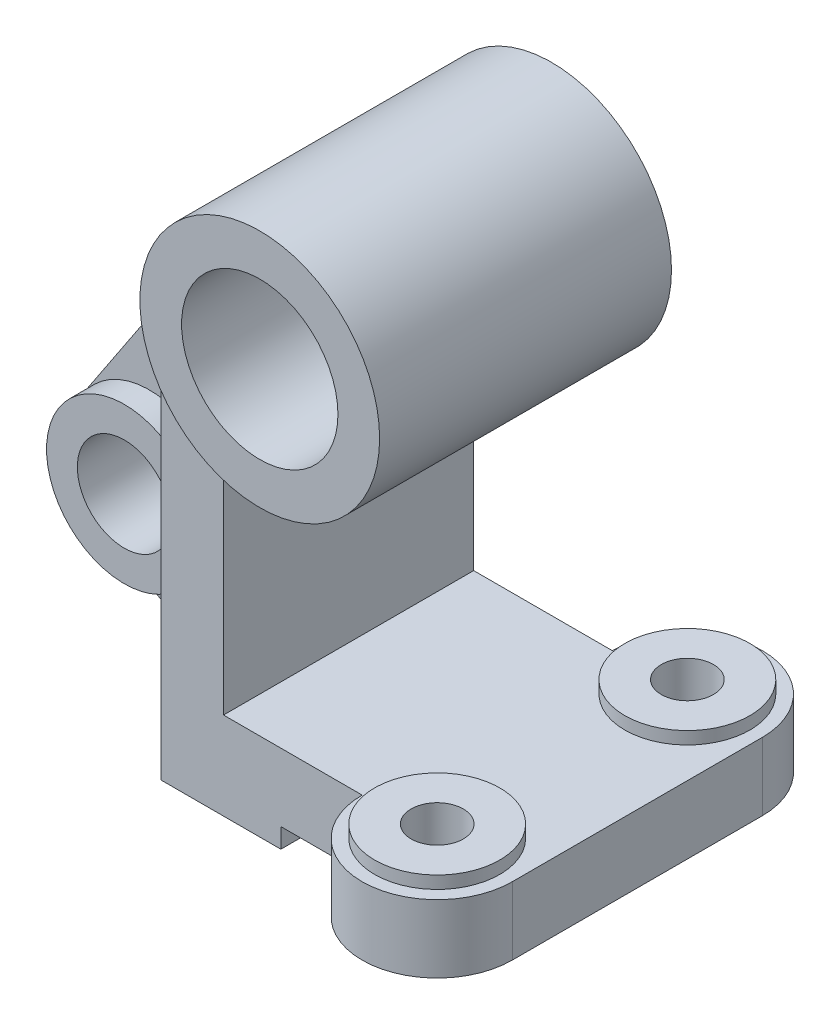
ISO-10303-21;
HEADER;
FILE_DESCRIPTION(('STEP AP214'),'2;1');
FILE_NAME('part.step','',(''),(''),'','','');
FILE_SCHEMA(('AUTOMOTIVE_DESIGN { 1 0 10303 214 1 1 1 1 }'));
ENDSEC;
DATA;
#1=APPLICATION_CONTEXT('core data for automotive mechanical design processes');
#2=APPLICATION_PROTOCOL_DEFINITION('international standard','automotive_design',2000,#1);
#3=PRODUCT_CONTEXT('',#1,'mechanical');
#4=PRODUCT('Part','Part','',(#3));
#5=PRODUCT_RELATED_PRODUCT_CATEGORY('part','',(#4));
#6=PRODUCT_DEFINITION_FORMATION('','',#4);
#7=PRODUCT_DEFINITION_CONTEXT('part definition',#1,'design');
#8=PRODUCT_DEFINITION('design','',#6,#7);
#9=PRODUCT_DEFINITION_SHAPE('','',#8);
#10=(LENGTH_UNIT() NAMED_UNIT(*) SI_UNIT(.MILLI.,.METRE.));
#11=(NAMED_UNIT(*) PLANE_ANGLE_UNIT() SI_UNIT($,.RADIAN.));
#12=(NAMED_UNIT(*) SI_UNIT($,.STERADIAN.) SOLID_ANGLE_UNIT());
#13=UNCERTAINTY_MEASURE_WITH_UNIT(LENGTH_MEASURE(1.E-05),#10,'distance_accuracy_value','');
#14=(GEOMETRIC_REPRESENTATION_CONTEXT(3) GLOBAL_UNCERTAINTY_ASSIGNED_CONTEXT((#13)) GLOBAL_UNIT_ASSIGNED_CONTEXT((#10,
#11,#12)) REPRESENTATION_CONTEXT('',''));
#15=CARTESIAN_POINT('',(0.,0.,0.));
#16=DIRECTION('',(0.,0.,1.));
#17=DIRECTION('',(1.,0.,0.));
#18=AXIS2_PLACEMENT_3D('',#15,#16,#17);
#19=CARTESIAN_POINT('',(67.1412556053812,0.,60.));
#20=DIRECTION('',(0.,1.,0.));
#21=DIRECTION('',(0.,0.,1.));
#22=AXIS2_PLACEMENT_3D('',#19,#20,#21);
#23=PLANE('',#22);
#24=DIRECTION('',(0.,0.,-1.));
#25=VECTOR('',#24,1.);
#26=CARTESIAN_POINT('',(-7.8587443946188,0.,145.));
#27=LINE('',#26,#25);
#28=CARTESIAN_POINT('',(-7.8587443946188,0.,60.));
#29=VERTEX_POINT('',#28);
#30=CARTESIAN_POINT('',(-7.8587443946188,0.,-60.));
#31=VERTEX_POINT('',#30);
#32=EDGE_CURVE('E160',#29,#31,#27,.T.);
#33=ORIENTED_EDGE('',*,*,#32,.F.);
#34=DIRECTION('',(1.,0.,0.));
#35=VECTOR('',#34,1.);
#36=CARTESIAN_POINT('',(-65.3587443946188,0.,60.));
#37=LINE('',#36,#35);
#38=CARTESIAN_POINT('',(-65.3587443946188,0.,60.));
#39=VERTEX_POINT('',#38);
#40=EDGE_CURVE('E317',#39,#29,#37,.T.);
#41=ORIENTED_EDGE('',*,*,#40,.F.);
#42=DIRECTION('',(0.,0.,1.));
#43=VECTOR('',#42,1.);
#44=CARTESIAN_POINT('',(-65.3587443946188,0.,-60.));
#45=LINE('',#44,#43);
#46=CARTESIAN_POINT('',(-65.3587443946188,0.,13.));
#47=VERTEX_POINT('',#46);
#48=EDGE_CURVE('E297',#47,#39,#45,.T.);
#49=ORIENTED_EDGE('',*,*,#48,.F.);
#50=DIRECTION('',(0.,0.,-1.));
#51=VECTOR('',#50,1.);
#52=CARTESIAN_POINT('',(-65.3587443946188,0.,13.));
#53=LINE('',#52,#51);
#54=CARTESIAN_POINT('',(-65.3587443946188,0.,-13.));
#55=VERTEX_POINT('',#54);
#56=EDGE_CURVE('E250',#47,#55,#53,.T.);
#57=ORIENTED_EDGE('',*,*,#56,.T.);
#58=CARTESIAN_POINT('',(-65.3587443946188,0.,-60.));
#59=VERTEX_POINT('',#58);
#60=EDGE_CURVE('E312',#59,#55,#45,.T.);
#61=ORIENTED_EDGE('',*,*,#60,.F.);
#62=DIRECTION('',(-1.,0.,0.));
#63=VECTOR('',#62,1.);
#64=CARTESIAN_POINT('',(-65.3587443946188,0.,-60.));
#65=LINE('',#64,#63);
#66=EDGE_CURVE('E302',#31,#59,#65,.T.);
#67=ORIENTED_EDGE('',*,*,#66,.F.);
#68=EDGE_LOOP('',(#33,#41,#49,#57,#61,#67));
#69=FACE_BOUND('',#68,.T.);
#70=ADVANCED_FACE('F41',(#69),#23,.F.);
#71=CARTESIAN_POINT('',(-65.3587443946188,42.,60.));
#72=DIRECTION('',(0.,0.,-1.));
#73=DIRECTION('',(-1.,0.,0.));
#74=AXIS2_PLACEMENT_3D('',#71,#72,#73);
#75=PLANE('',#74);
#76=DIRECTION('',(0.,-1.,0.));
#77=VECTOR('',#76,1.);
#78=CARTESIAN_POINT('',(-7.8587443946188,42.,60.));
#79=LINE('',#78,#77);
#80=CARTESIAN_POINT('',(-7.8587443946188,9.41903160837437,60.));
#81=VERTEX_POINT('',#80);
#82=EDGE_CURVE('E201',#81,#29,#79,.T.);
#83=ORIENTED_EDGE('',*,*,#82,.F.);
#84=DIRECTION('',(-1.,0.,0.));
#85=VECTOR('',#84,1.);
#86=CARTESIAN_POINT('',(-65.3587443946188,9.41903160837437,60.));
#87=LINE('',#86,#85);
#88=CARTESIAN_POINT('',(31.1412556053812,9.41903160837437,60.));
#89=VERTEX_POINT('',#88);
#90=EDGE_CURVE('E166',#89,#81,#87,.T.);
#91=ORIENTED_EDGE('',*,*,#90,.F.);
#92=DIRECTION('',(0.,-1.,0.));
#93=VECTOR('',#92,1.);
#94=CARTESIAN_POINT('',(31.1412556053812,42.,60.));
#95=LINE('',#94,#93);
#96=CARTESIAN_POINT('',(31.1412556053812,42.,60.));
#97=VERTEX_POINT('',#96);
#98=EDGE_CURVE('E170',#97,#89,#95,.T.);
#99=ORIENTED_EDGE('',*,*,#98,.F.);
#100=DIRECTION('',(1.,0.,0.));
#101=VECTOR('',#100,1.);
#102=CARTESIAN_POINT('',(-65.3587443946188,42.,60.));
#103=LINE('',#102,#101);
#104=CARTESIAN_POINT('',(-35.3587443946188,42.,60.));
#105=VERTEX_POINT('',#104);
#106=EDGE_CURVE('E301',#105,#97,#103,.T.);
#107=ORIENTED_EDGE('',*,*,#106,.F.);
#108=DIRECTION('',(0.,-1.,0.));
#109=VECTOR('',#108,1.);
#110=CARTESIAN_POINT('',(-35.3587443946188,208.,60.));
#111=LINE('',#110,#109);
#112=CARTESIAN_POINT('',(-35.3587443946188,153.774019557073,60.));
#113=VERTEX_POINT('',#112);
#114=EDGE_CURVE('E296',#113,#105,#111,.T.);
#115=ORIENTED_EDGE('',*,*,#114,.F.);
#116=CARTESIAN_POINT('',(-7.9756626414212,204.335040449631,60.));
#117=DIRECTION('',(0.,0.,-1.));
#118=DIRECTION('',(-1.,0.,0.));
#119=AXIS2_PLACEMENT_3D('',#116,#117,#118);
#120=CIRCLE('',#119,57.5);
#121=CARTESIAN_POINT('',(-65.3587443946188,200.670080899262,60.));
#122=VERTEX_POINT('',#121);
#123=EDGE_CURVE('E290',#122,#113,#120,.F.);
#124=ORIENTED_EDGE('',*,*,#123,.F.);
#125=DIRECTION('',(0.,-1.,0.));
#126=VECTOR('',#125,1.);
#127=CARTESIAN_POINT('',(-65.3587443946188,42.,60.));
#128=LINE('',#127,#126);
#129=EDGE_CURVE('E172',#122,#39,#128,.T.);
#130=ORIENTED_EDGE('',*,*,#129,.T.);
#131=ORIENTED_EDGE('',*,*,#40,.T.);
#132=EDGE_LOOP('',(#83,#91,#99,#107,#115,#124,#130,#131));
#133=FACE_BOUND('',#132,.T.);
#134=ADVANCED_FACE('F336',(#133),#75,.F.);
#135=CARTESIAN_POINT('',(67.1412556053812,42.,60.));
#136=DIRECTION('',(0.,-1.,0.));
#137=DIRECTION('',(0.,0.,-1.));
#138=AXIS2_PLACEMENT_3D('',#135,#136,#137);
#139=CYLINDRICAL_SURFACE('',#138,36.);
#140=CARTESIAN_POINT('',(67.1412556053812,9.41903160837437,60.));
#141=DIRECTION('',(0.,-1.,0.));
#142=DIRECTION('',(0.,0.,-1.));
#143=AXIS2_PLACEMENT_3D('',#140,#141,#142);
#144=CIRCLE('',#143,36.);
#145=CARTESIAN_POINT('',(103.141255605381,9.41903160837437,60.));
#146=VERTEX_POINT('',#145);
#147=EDGE_CURVE('E148',#146,#89,#144,.T.);
#148=ORIENTED_EDGE('',*,*,#147,.F.);
#149=DIRECTION('',(0.,-1.,0.));
#150=VECTOR('',#149,1.);
#151=CARTESIAN_POINT('',(103.141255605381,42.,60.));
#152=LINE('',#151,#150);
#153=CARTESIAN_POINT('',(103.141255605381,42.,60.));
#154=VERTEX_POINT('',#153);
#155=EDGE_CURVE('E165',#154,#146,#152,.T.);
#156=ORIENTED_EDGE('',*,*,#155,.F.);
#157=CARTESIAN_POINT('',(67.1412556053812,42.,60.));
#158=DIRECTION('',(0.,1.,0.));
#159=DIRECTION('',(0.,0.,1.));
#160=AXIS2_PLACEMENT_3D('',#157,#158,#159);
#161=CIRCLE('',#160,36.);
#162=EDGE_CURVE('E303',#97,#154,#161,.T.);
#163=ORIENTED_EDGE('',*,*,#162,.F.);
#164=ORIENTED_EDGE('',*,*,#98,.T.);
#165=EDGE_LOOP('',(#148,#156,#163,#164));
#166=FACE_BOUND('',#165,.T.);
#167=ADVANCED_FACE('F162',(#166),#139,.T.);
#168=CARTESIAN_POINT('',(103.141255605381,42.,-60.));
#169=DIRECTION('',(-1.,0.,0.));
#170=DIRECTION('',(0.,0.,1.));
#171=AXIS2_PLACEMENT_3D('',#168,#169,#170);
#172=PLANE('',#171);
#173=DIRECTION('',(0.,0.,-1.));
#174=VECTOR('',#173,1.);
#175=CARTESIAN_POINT('',(103.141255605381,9.41903160837437,145.));
#176=LINE('',#175,#174);
#177=CARTESIAN_POINT('',(103.141255605381,9.41903160837437,-60.));
#178=VERTEX_POINT('',#177);
#179=EDGE_CURVE('E149',#146,#178,#176,.T.);
#180=ORIENTED_EDGE('',*,*,#179,.T.);
#181=DIRECTION('',(0.,-1.,0.));
#182=VECTOR('',#181,1.);
#183=CARTESIAN_POINT('',(103.141255605381,42.,-60.));
#184=LINE('',#183,#182);
#185=CARTESIAN_POINT('',(103.141255605381,42.,-60.));
#186=VERTEX_POINT('',#185);
#187=EDGE_CURVE('E175',#186,#178,#184,.T.);
#188=ORIENTED_EDGE('',*,*,#187,.F.);
#189=DIRECTION('',(0.,0.,-1.));
#190=VECTOR('',#189,1.);
#191=CARTESIAN_POINT('',(103.141255605381,42.,-60.));
#192=LINE('',#191,#190);
#193=EDGE_CURVE('E171',#154,#186,#192,.T.);
#194=ORIENTED_EDGE('',*,*,#193,.F.);
#195=ORIENTED_EDGE('',*,*,#155,.T.);
#196=EDGE_LOOP('',(#180,#188,#194,#195));
#197=FACE_BOUND('',#196,.T.);
#198=ADVANCED_FACE('F167',(#197),#172,.F.);
#199=CARTESIAN_POINT('',(67.1412556053812,42.,-60.));
#200=DIRECTION('',(0.,-1.,0.));
#201=DIRECTION('',(0.,0.,-1.));
#202=AXIS2_PLACEMENT_3D('',#199,#200,#201);
#203=CYLINDRICAL_SURFACE('',#202,36.);
#204=CARTESIAN_POINT('',(67.1412556053812,9.41903160837437,-60.));
#205=DIRECTION('',(0.,-1.,0.));
#206=DIRECTION('',(0.,0.,-1.));
#207=AXIS2_PLACEMENT_3D('',#204,#205,#206);
#208=CIRCLE('',#207,36.);
#209=CARTESIAN_POINT('',(31.1412556053812,9.41903160837437,-60.));
#210=VERTEX_POINT('',#209);
#211=EDGE_CURVE('E155',#210,#178,#208,.T.);
#212=ORIENTED_EDGE('',*,*,#211,.F.);
#213=DIRECTION('',(0.,-1.,0.));
#214=VECTOR('',#213,1.);
#215=CARTESIAN_POINT('',(31.1412556053812,42.,-60.));
#216=LINE('',#215,#214);
#217=CARTESIAN_POINT('',(31.1412556053812,42.,-60.));
#218=VERTEX_POINT('',#217);
#219=EDGE_CURVE('E176',#218,#210,#216,.T.);
#220=ORIENTED_EDGE('',*,*,#219,.F.);
#221=CARTESIAN_POINT('',(67.1412556053812,42.,-60.));
#222=DIRECTION('',(0.,1.,0.));
#223=DIRECTION('',(0.,0.,-1.));
#224=AXIS2_PLACEMENT_3D('',#221,#222,#223);
#225=CIRCLE('',#224,36.);
#226=EDGE_CURVE('E310',#186,#218,#225,.T.);
#227=ORIENTED_EDGE('',*,*,#226,.F.);
#228=ORIENTED_EDGE('',*,*,#187,.T.);
#229=EDGE_LOOP('',(#212,#220,#227,#228));
#230=FACE_BOUND('',#229,.T.);
#231=ADVANCED_FACE('F327',(#230),#203,.T.);
#232=CARTESIAN_POINT('',(-65.3587443946188,42.,-60.));
#233=DIRECTION('',(0.,0.,1.));
#234=DIRECTION('',(1.,0.,0.));
#235=AXIS2_PLACEMENT_3D('',#232,#233,#234);
#236=PLANE('',#235);
#237=DIRECTION('',(0.,1.,0.));
#238=VECTOR('',#237,1.);
#239=CARTESIAN_POINT('',(-7.8587443946188,42.,-60.));
#240=LINE('',#239,#238);
#241=CARTESIAN_POINT('',(-7.8587443946188,9.41903160837437,-60.));
#242=VERTEX_POINT('',#241);
#243=EDGE_CURVE('E11',#31,#242,#240,.T.);
#244=ORIENTED_EDGE('',*,*,#243,.F.);
#245=ORIENTED_EDGE('',*,*,#66,.T.);
#246=DIRECTION('',(0.,-1.,0.));
#247=VECTOR('',#246,1.);
#248=CARTESIAN_POINT('',(-65.3587443946188,42.,-60.));
#249=LINE('',#248,#247);
#250=CARTESIAN_POINT('',(-65.3587443946188,200.670080899262,-60.));
#251=VERTEX_POINT('',#250);
#252=EDGE_CURVE('E315',#251,#59,#249,.T.);
#253=ORIENTED_EDGE('',*,*,#252,.F.);
#254=CARTESIAN_POINT('',(-7.9756626414212,204.335040449631,-60.));
#255=DIRECTION('',(0.,0.,1.));
#256=DIRECTION('',(1.,0.,0.));
#257=AXIS2_PLACEMENT_3D('',#254,#255,#256);
#258=CIRCLE('',#257,57.5);
#259=CARTESIAN_POINT('',(-35.3587443946188,153.774019557073,-60.));
#260=VERTEX_POINT('',#259);
#261=EDGE_CURVE('E282',#260,#251,#258,.F.);
#262=ORIENTED_EDGE('',*,*,#261,.F.);
#263=DIRECTION('',(0.,-1.,0.));
#264=VECTOR('',#263,1.);
#265=CARTESIAN_POINT('',(-35.3587443946188,208.,-60.));
#266=LINE('',#265,#264);
#267=CARTESIAN_POINT('',(-35.3587443946188,42.,-60.));
#268=VERTEX_POINT('',#267);
#269=EDGE_CURVE('E298',#260,#268,#266,.T.);
#270=ORIENTED_EDGE('',*,*,#269,.T.);
#271=DIRECTION('',(-1.,0.,0.));
#272=VECTOR('',#271,1.);
#273=CARTESIAN_POINT('',(-65.3587443946188,42.,-60.));
#274=LINE('',#273,#272);
#275=EDGE_CURVE('E307',#218,#268,#274,.T.);
#276=ORIENTED_EDGE('',*,*,#275,.F.);
#277=ORIENTED_EDGE('',*,*,#219,.T.);
#278=DIRECTION('',(1.,0.,0.));
#279=VECTOR('',#278,1.);
#280=CARTESIAN_POINT('',(-65.3587443946188,9.41903160837437,-60.));
#281=LINE('',#280,#279);
#282=EDGE_CURVE('E191',#242,#210,#281,.T.);
#283=ORIENTED_EDGE('',*,*,#282,.F.);
#284=EDGE_LOOP('',(#244,#245,#253,#262,#270,#276,#277,#283));
#285=FACE_BOUND('',#284,.T.);
#286=ADVANCED_FACE('F326',(#285),#236,.F.);
#287=CARTESIAN_POINT('',(67.1412556053812,42.,60.));
#288=DIRECTION('',(0.,-1.,0.));
#289=DIRECTION('',(0.,0.,-1.));
#290=AXIS2_PLACEMENT_3D('',#287,#288,#289);
#291=CYLINDRICAL_SURFACE('',#290,12.5);
#292=CARTESIAN_POINT('',(67.1412556053812,48.,60.));
#293=DIRECTION('',(0.,1.,0.));
#294=DIRECTION('',(0.,0.,1.));
#295=AXIS2_PLACEMENT_3D('',#292,#293,#294);
#296=CIRCLE('',#295,12.5);
#297=CARTESIAN_POINT('',(67.1412556053812,48.,47.5));
#298=VERTEX_POINT('',#297);
#299=EDGE_CURVE('E211',#298,#298,#296,.T.);
#300=CARTESIAN_POINT('',(67.1412556053812,9.41903160837437,60.));
#301=DIRECTION('',(0.,-1.,0.));
#302=DIRECTION('',(0.,0.,-1.));
#303=AXIS2_PLACEMENT_3D('',#300,#301,#302);
#304=CIRCLE('',#303,12.5);
#305=CARTESIAN_POINT('',(67.1412556053812,9.41903160837437,47.5));
#306=VERTEX_POINT('',#305);
#307=EDGE_CURVE('E189',#306,#306,#304,.T.);
#308=CARTESIAN_POINT('',(67.1412556053812,48.,47.5));
#309=CARTESIAN_POINT('',(67.1412556053812,47.5981149125872,47.5));
#310=CARTESIAN_POINT('',(67.1412556053812,47.1962298251745,47.5));
#311=CARTESIAN_POINT('',(67.1412556053812,46.3924596503489,47.5));
#312=CARTESIAN_POINT('',(67.1412556053812,45.9905745629362,47.5));
#313=CARTESIAN_POINT('',(67.1412556053812,45.1868043881106,47.5));
#314=CARTESIAN_POINT('',(67.1412556053812,44.7849193006979,47.5));
#315=CARTESIAN_POINT('',(67.1412556053812,43.9811491258723,47.5));
#316=CARTESIAN_POINT('',(67.1412556053812,43.5792640384596,47.5));
#317=CARTESIAN_POINT('',(67.1412556053812,42.775493863634,47.5));
#318=CARTESIAN_POINT('',(67.1412556053812,42.3736087762213,47.5));
#319=CARTESIAN_POINT('',(67.1412556053812,41.5698386013957,47.5));
#320=CARTESIAN_POINT('',(67.1412556053812,41.167953513983,47.5));
#321=CARTESIAN_POINT('',(67.1412556053812,40.3641833391574,47.5));
#322=CARTESIAN_POINT('',(67.1412556053812,39.9622982517447,47.5));
#323=CARTESIAN_POINT('',(67.1412556053812,39.1585280769191,47.5));
#324=CARTESIAN_POINT('',(67.1412556053812,38.7566429895064,47.5));
#325=CARTESIAN_POINT('',(67.1412556053812,37.9528728146808,47.5));
#326=CARTESIAN_POINT('',(67.1412556053812,37.5509877272681,47.5));
#327=CARTESIAN_POINT('',(67.1412556053812,36.7472175524425,47.5));
#328=CARTESIAN_POINT('',(67.1412556053812,36.3453324650298,47.5));
#329=CARTESIAN_POINT('',(67.1412556053812,35.5415622902042,47.5));
#330=CARTESIAN_POINT('',(67.1412556053812,35.1396772027915,47.5));
#331=CARTESIAN_POINT('',(67.1412556053812,34.3359070279659,47.5));
#332=CARTESIAN_POINT('',(67.1412556053812,33.9340219405532,47.5));
#333=CARTESIAN_POINT('',(67.1412556053812,33.1302517657276,47.5));
#334=CARTESIAN_POINT('',(67.1412556053812,32.7283666783149,47.5));
#335=CARTESIAN_POINT('',(67.1412556053812,31.9245965034893,47.5));
#336=CARTESIAN_POINT('',(67.1412556053812,31.5227114160766,47.5));
#337=CARTESIAN_POINT('',(67.1412556053812,30.718941241251,47.5));
#338=CARTESIAN_POINT('',(67.1412556053812,30.3170561538383,47.5));
#339=CARTESIAN_POINT('',(67.1412556053812,29.5132859790127,47.5));
#340=CARTESIAN_POINT('',(67.1412556053812,29.1114008916,47.5));
#341=CARTESIAN_POINT('',(67.1412556053812,28.3076307167744,47.5));
#342=CARTESIAN_POINT('',(67.1412556053812,27.9057456293617,47.5));
#343=CARTESIAN_POINT('',(67.1412556053812,27.1019754545361,47.5));
#344=CARTESIAN_POINT('',(67.1412556053812,26.7000903671234,47.5));
#345=CARTESIAN_POINT('',(67.1412556053812,25.8963201922978,47.5));
#346=CARTESIAN_POINT('',(67.1412556053812,25.4944351048851,47.5));
#347=CARTESIAN_POINT('',(67.1412556053812,24.6906649300595,47.5));
#348=CARTESIAN_POINT('',(67.1412556053812,24.2887798426468,47.5));
#349=CARTESIAN_POINT('',(67.1412556053812,23.4850096678212,47.5));
#350=CARTESIAN_POINT('',(67.1412556053812,23.0831245804085,47.5));
#351=CARTESIAN_POINT('',(67.1412556053812,22.2793544055829,47.5));
#352=CARTESIAN_POINT('',(67.1412556053812,21.8774693181701,47.5));
#353=CARTESIAN_POINT('',(67.1412556053812,21.0736991433446,47.5));
#354=CARTESIAN_POINT('',(67.1412556053812,20.6718140559318,47.5));
#355=CARTESIAN_POINT('',(67.1412556053812,19.8680438811063,47.5));
#356=CARTESIAN_POINT('',(67.1412556053812,19.4661587936935,47.5));
#357=CARTESIAN_POINT('',(67.1412556053812,18.662388618868,47.5));
#358=CARTESIAN_POINT('',(67.1412556053812,18.2605035314552,47.5));
#359=CARTESIAN_POINT('',(67.1412556053812,17.4567333566297,47.5));
#360=CARTESIAN_POINT('',(67.1412556053812,17.0548482692169,47.5));
#361=CARTESIAN_POINT('',(67.1412556053812,16.2510780943914,47.5));
#362=CARTESIAN_POINT('',(67.1412556053812,15.8491930069786,47.5));
#363=CARTESIAN_POINT('',(67.1412556053812,15.0454228321531,47.5));
#364=CARTESIAN_POINT('',(67.1412556053812,14.6435377447403,47.5));
#365=CARTESIAN_POINT('',(67.1412556053812,13.8397675699148,47.5));
#366=CARTESIAN_POINT('',(67.1412556053812,13.437882482502,47.5));
#367=CARTESIAN_POINT('',(67.1412556053812,12.6341123076765,47.5));
#368=CARTESIAN_POINT('',(67.1412556053812,12.2322272202637,47.5));
#369=CARTESIAN_POINT('',(67.1412556053812,11.4284570454382,47.5));
#370=CARTESIAN_POINT('',(67.1412556053812,11.0265719580254,47.5));
#371=CARTESIAN_POINT('',(67.1412556053812,10.2228017831999,47.5));
#372=CARTESIAN_POINT('',(67.1412556053812,9.82091669578714,47.5));
#373=CARTESIAN_POINT('',(67.1412556053812,9.41903160837437,47.5));
#374=B_SPLINE_CURVE_WITH_KNOTS('',3,(#308,#309,#310,#311,#312,#313,#314,#315,#316,#317,#318,
#319,#320,#321,#322,#323,#324,#325,#326,#327,#328,#329,#330,#331,#332,#333,#334,#335,#336,#337,
#338,#339,#340,#341,#342,#343,#344,#345,#346,#347,#348,#349,#350,#351,#352,#353,#354,#355,#356,
#357,#358,#359,#360,#361,#362,#363,#364,#365,#366,#367,#368,#369,#370,#371,#372,#373),
.UNSPECIFIED.,.F.,.F.,(4,2,2,2,2,2,2,2,2,2,2,2,2,2,2,2,2,2,2,2,2,2,2,2,2,2,2,2,2,2,2,2,4),(0.,
1.2056552622383,2.4113105244766,3.6169657867149,4.8226210489532,6.0282763111915,7.2339315734298,
8.4395868356681,9.6452420979064,10.8508973601447,12.056552622383,13.2622078846213,
14.4678631468596,15.6735184090979,16.8791736713362,18.0848289335745,19.2904841958128,
20.4961394580511,21.7017947202894,22.9074499825277,24.113105244766,25.3187605070043,
26.5244157692426,27.7300710314809,28.9357262937192,30.1413815559575,31.3470368181958,
32.5526920804341,33.7583473426724,34.9640026049107,36.169657867149,37.3753131293873,
38.5809683916256),.UNSPECIFIED.);
#375=EDGE_CURVE('BSEAM395',#298,#306,#374,.T.);
#376=ORIENTED_EDGE('',*,*,#299,.T.);
#377=ORIENTED_EDGE('',*,*,#307,.T.);
#378=ORIENTED_EDGE('',*,*,#375,.T.);
#379=ORIENTED_EDGE('',*,*,#375,.F.);
#380=EDGE_LOOP('',(#376,#378,#377,#379));
#381=FACE_BOUND('',#380,.T.);
#382=ADVANCED_FACE('F395',(#381),#291,.F.);
#383=CARTESIAN_POINT('',(67.1412556053812,42.,-60.));
#384=DIRECTION('',(0.,-1.,0.));
#385=DIRECTION('',(0.,0.,-1.));
#386=AXIS2_PLACEMENT_3D('',#383,#384,#385);
#387=CYLINDRICAL_SURFACE('',#386,12.5);
#388=CARTESIAN_POINT('',(67.1412556053812,48.,-60.));
#389=DIRECTION('',(0.,1.,0.));
#390=DIRECTION('',(0.,0.,1.));
#391=AXIS2_PLACEMENT_3D('',#388,#389,#390);
#392=CIRCLE('',#391,12.5);
#393=CARTESIAN_POINT('',(67.1412556053812,48.,-72.5));
#394=VERTEX_POINT('',#393);
#395=EDGE_CURVE('E202',#394,#394,#392,.T.);
#396=CARTESIAN_POINT('',(67.1412556053812,9.41903160837437,-60.));
#397=DIRECTION('',(0.,-1.,0.));
#398=DIRECTION('',(0.,0.,-1.));
#399=AXIS2_PLACEMENT_3D('',#396,#397,#398);
#400=CIRCLE('',#399,12.5);
#401=CARTESIAN_POINT('',(67.1412556053812,9.41903160837437,-72.5));
#402=VERTEX_POINT('',#401);
#403=EDGE_CURVE('E187',#402,#402,#400,.T.);
#404=CARTESIAN_POINT('',(67.1412556053812,48.,-72.5));
#405=CARTESIAN_POINT('',(67.1412556053812,47.5981149125872,-72.5));
#406=CARTESIAN_POINT('',(67.1412556053812,47.1962298251745,-72.5));
#407=CARTESIAN_POINT('',(67.1412556053812,46.3924596503489,-72.5));
#408=CARTESIAN_POINT('',(67.1412556053812,45.9905745629362,-72.5));
#409=CARTESIAN_POINT('',(67.1412556053812,45.1868043881106,-72.5));
#410=CARTESIAN_POINT('',(67.1412556053812,44.7849193006979,-72.5));
#411=CARTESIAN_POINT('',(67.1412556053812,43.9811491258723,-72.5));
#412=CARTESIAN_POINT('',(67.1412556053812,43.5792640384596,-72.5));
#413=CARTESIAN_POINT('',(67.1412556053812,42.775493863634,-72.5));
#414=CARTESIAN_POINT('',(67.1412556053812,42.3736087762213,-72.5));
#415=CARTESIAN_POINT('',(67.1412556053812,41.5698386013957,-72.5));
#416=CARTESIAN_POINT('',(67.1412556053812,41.167953513983,-72.5));
#417=CARTESIAN_POINT('',(67.1412556053812,40.3641833391574,-72.5));
#418=CARTESIAN_POINT('',(67.1412556053812,39.9622982517447,-72.5));
#419=CARTESIAN_POINT('',(67.1412556053812,39.1585280769191,-72.5));
#420=CARTESIAN_POINT('',(67.1412556053812,38.7566429895064,-72.5));
#421=CARTESIAN_POINT('',(67.1412556053812,37.9528728146808,-72.5));
#422=CARTESIAN_POINT('',(67.1412556053812,37.5509877272681,-72.5));
#423=CARTESIAN_POINT('',(67.1412556053812,36.7472175524425,-72.5));
#424=CARTESIAN_POINT('',(67.1412556053812,36.3453324650298,-72.5));
#425=CARTESIAN_POINT('',(67.1412556053812,35.5415622902042,-72.5));
#426=CARTESIAN_POINT('',(67.1412556053812,35.1396772027915,-72.5));
#427=CARTESIAN_POINT('',(67.1412556053812,34.3359070279659,-72.5));
#428=CARTESIAN_POINT('',(67.1412556053812,33.9340219405532,-72.5));
#429=CARTESIAN_POINT('',(67.1412556053812,33.1302517657276,-72.5));
#430=CARTESIAN_POINT('',(67.1412556053812,32.7283666783149,-72.5));
#431=CARTESIAN_POINT('',(67.1412556053812,31.9245965034893,-72.5));
#432=CARTESIAN_POINT('',(67.1412556053812,31.5227114160766,-72.5));
#433=CARTESIAN_POINT('',(67.1412556053812,30.718941241251,-72.5));
#434=CARTESIAN_POINT('',(67.1412556053812,30.3170561538383,-72.5));
#435=CARTESIAN_POINT('',(67.1412556053812,29.5132859790127,-72.5));
#436=CARTESIAN_POINT('',(67.1412556053812,29.1114008916,-72.5));
#437=CARTESIAN_POINT('',(67.1412556053812,28.3076307167744,-72.5));
#438=CARTESIAN_POINT('',(67.1412556053812,27.9057456293617,-72.5));
#439=CARTESIAN_POINT('',(67.1412556053812,27.1019754545361,-72.5));
#440=CARTESIAN_POINT('',(67.1412556053812,26.7000903671234,-72.5));
#441=CARTESIAN_POINT('',(67.1412556053812,25.8963201922978,-72.5));
#442=CARTESIAN_POINT('',(67.1412556053812,25.4944351048851,-72.5));
#443=CARTESIAN_POINT('',(67.1412556053812,24.6906649300595,-72.5));
#444=CARTESIAN_POINT('',(67.1412556053812,24.2887798426468,-72.5));
#445=CARTESIAN_POINT('',(67.1412556053812,23.4850096678212,-72.5));
#446=CARTESIAN_POINT('',(67.1412556053812,23.0831245804085,-72.5));
#447=CARTESIAN_POINT('',(67.1412556053812,22.2793544055829,-72.5));
#448=CARTESIAN_POINT('',(67.1412556053812,21.8774693181701,-72.5));
#449=CARTESIAN_POINT('',(67.1412556053812,21.0736991433446,-72.5));
#450=CARTESIAN_POINT('',(67.1412556053812,20.6718140559318,-72.5));
#451=CARTESIAN_POINT('',(67.1412556053812,19.8680438811063,-72.5));
#452=CARTESIAN_POINT('',(67.1412556053812,19.4661587936935,-72.5));
#453=CARTESIAN_POINT('',(67.1412556053812,18.662388618868,-72.5));
#454=CARTESIAN_POINT('',(67.1412556053812,18.2605035314552,-72.5));
#455=CARTESIAN_POINT('',(67.1412556053812,17.4567333566297,-72.5));
#456=CARTESIAN_POINT('',(67.1412556053812,17.0548482692169,-72.5));
#457=CARTESIAN_POINT('',(67.1412556053812,16.2510780943914,-72.5));
#458=CARTESIAN_POINT('',(67.1412556053812,15.8491930069786,-72.5));
#459=CARTESIAN_POINT('',(67.1412556053812,15.0454228321531,-72.5));
#460=CARTESIAN_POINT('',(67.1412556053812,14.6435377447403,-72.5));
#461=CARTESIAN_POINT('',(67.1412556053812,13.8397675699148,-72.5));
#462=CARTESIAN_POINT('',(67.1412556053812,13.437882482502,-72.5));
#463=CARTESIAN_POINT('',(67.1412556053812,12.6341123076765,-72.5));
#464=CARTESIAN_POINT('',(67.1412556053812,12.2322272202637,-72.5));
#465=CARTESIAN_POINT('',(67.1412556053812,11.4284570454382,-72.5));
#466=CARTESIAN_POINT('',(67.1412556053812,11.0265719580254,-72.5));
#467=CARTESIAN_POINT('',(67.1412556053812,10.2228017831999,-72.5));
#468=CARTESIAN_POINT('',(67.1412556053812,9.82091669578714,-72.5));
#469=CARTESIAN_POINT('',(67.1412556053812,9.41903160837437,-72.5));
#470=B_SPLINE_CURVE_WITH_KNOTS('',3,(#404,#405,#406,#407,#408,#409,#410,#411,#412,#413,#414,
#415,#416,#417,#418,#419,#420,#421,#422,#423,#424,#425,#426,#427,#428,#429,#430,#431,#432,#433,
#434,#435,#436,#437,#438,#439,#440,#441,#442,#443,#444,#445,#446,#447,#448,#449,#450,#451,#452,
#453,#454,#455,#456,#457,#458,#459,#460,#461,#462,#463,#464,#465,#466,#467,#468,#469),
.UNSPECIFIED.,.F.,.F.,(4,2,2,2,2,2,2,2,2,2,2,2,2,2,2,2,2,2,2,2,2,2,2,2,2,2,2,2,2,2,2,2,4),(0.,
1.2056552622383,2.4113105244766,3.6169657867149,4.8226210489532,6.0282763111915,7.2339315734298,
8.4395868356681,9.6452420979064,10.8508973601447,12.056552622383,13.2622078846213,
14.4678631468596,15.6735184090979,16.8791736713362,18.0848289335745,19.2904841958128,
20.4961394580511,21.7017947202894,22.9074499825277,24.113105244766,25.3187605070043,
26.5244157692426,27.7300710314809,28.9357262937192,30.1413815559575,31.3470368181958,
32.5526920804341,33.7583473426724,34.9640026049107,36.169657867149,37.3753131293873,
38.5809683916256),.UNSPECIFIED.);
#471=EDGE_CURVE('BSEAM417',#394,#402,#470,.T.);
#472=ORIENTED_EDGE('',*,*,#395,.T.);
#473=ORIENTED_EDGE('',*,*,#403,.T.);
#474=ORIENTED_EDGE('',*,*,#471,.T.);
#475=ORIENTED_EDGE('',*,*,#471,.F.);
#476=EDGE_LOOP('',(#472,#474,#473,#475));
#477=FACE_BOUND('',#476,.T.);
#478=ADVANCED_FACE('F417',(#477),#387,.F.);
#479=CARTESIAN_POINT('',(67.1412556053812,42.,60.));
#480=DIRECTION('',(0.,1.,0.));
#481=DIRECTION('',(0.,0.,1.));
#482=AXIS2_PLACEMENT_3D('',#479,#480,#481);
#483=PLANE('',#482);
#484=CARTESIAN_POINT('',(67.1412556053812,42.,60.));
#485=DIRECTION('',(0.,1.,0.));
#486=DIRECTION('',(0.,0.,1.));
#487=AXIS2_PLACEMENT_3D('',#484,#485,#486);
#488=CIRCLE('',#487,30.);
#489=CARTESIAN_POINT('',(67.1412556053812,42.,90.));
#490=VERTEX_POINT('',#489);
#491=EDGE_CURVE('E220',#490,#490,#488,.T.);
#492=ORIENTED_EDGE('',*,*,#491,.F.);
#493=EDGE_LOOP('',(#492));
#494=FACE_BOUND('',#493,.T.);
#495=DIRECTION('',(0.,0.,-1.));
#496=VECTOR('',#495,1.);
#497=CARTESIAN_POINT('',(-35.3587443946188,42.,-60.));
#498=LINE('',#497,#496);
#499=EDGE_CURVE('E291',#105,#268,#498,.T.);
#500=ORIENTED_EDGE('',*,*,#499,.F.);
#501=ORIENTED_EDGE('',*,*,#106,.T.);
#502=ORIENTED_EDGE('',*,*,#162,.T.);
#503=ORIENTED_EDGE('',*,*,#193,.T.);
#504=ORIENTED_EDGE('',*,*,#226,.T.);
#505=ORIENTED_EDGE('',*,*,#275,.T.);
#506=EDGE_LOOP('',(#500,#501,#502,#503,#504,#505));
#507=FACE_BOUND('',#506,.T.);
#508=CARTESIAN_POINT('',(67.1412556053812,42.,-60.));
#509=DIRECTION('',(0.,1.,0.));
#510=DIRECTION('',(0.,0.,1.));
#511=AXIS2_PLACEMENT_3D('',#508,#509,#510);
#512=CIRCLE('',#511,30.);
#513=CARTESIAN_POINT('',(67.1412556053812,42.,-30.));
#514=VERTEX_POINT('',#513);
#515=EDGE_CURVE('E206',#514,#514,#512,.T.);
#516=ORIENTED_EDGE('',*,*,#515,.F.);
#517=EDGE_LOOP('',(#516));
#518=FACE_BOUND('',#517,.T.);
#519=ADVANCED_FACE('F335',(#494,#507,#518),#483,.T.);
#520=CARTESIAN_POINT('',(-65.3587443946188,42.,-60.));
#521=DIRECTION('',(1.,0.,0.));
#522=DIRECTION('',(0.,0.,-1.));
#523=AXIS2_PLACEMENT_3D('',#520,#521,#522);
#524=PLANE('',#523);
#525=DIRECTION('',(0.,-1.,0.));
#526=VECTOR('',#525,1.);
#527=CARTESIAN_POINT('',(-65.3587443946188,0.,-13.));
#528=LINE('',#527,#526);
#529=CARTESIAN_POINT('',(-65.3587443946188,200.670080899262,-13.));
#530=VERTEX_POINT('',#529);
#531=EDGE_CURVE('E237',#530,#55,#528,.T.);
#532=ORIENTED_EDGE('',*,*,#531,.F.);
#533=DIRECTION('',(0.,0.,-1.));
#534=VECTOR('',#533,1.);
#535=CARTESIAN_POINT('',(-65.3587443946188,200.670080899262,70.));
#536=LINE('',#535,#534);
#537=EDGE_CURVE('E293',#251,#530,#536,.F.);
#538=ORIENTED_EDGE('',*,*,#537,.F.);
#539=ORIENTED_EDGE('',*,*,#252,.T.);
#540=ORIENTED_EDGE('',*,*,#60,.T.);
#541=EDGE_LOOP('',(#532,#538,#539,#540));
#542=FACE_BOUND('',#541,.T.);
#543=ADVANCED_FACE('F348',(#542),#524,.F.);
#544=CARTESIAN_POINT('',(-65.3587443946188,200.670080899262,13.));
#545=VERTEX_POINT('',#544);
#546=EDGE_CURVE('E287',#545,#122,#536,.F.);
#547=ORIENTED_EDGE('',*,*,#546,.F.);
#548=DIRECTION('',(0.,-1.,0.));
#549=VECTOR('',#548,1.);
#550=CARTESIAN_POINT('',(-65.3587443946188,0.,13.));
#551=LINE('',#550,#549);
#552=EDGE_CURVE('E65',#545,#47,#551,.T.);
#553=ORIENTED_EDGE('',*,*,#552,.T.);
#554=ORIENTED_EDGE('',*,*,#48,.T.);
#555=ORIENTED_EDGE('',*,*,#129,.F.);
#556=EDGE_LOOP('',(#547,#553,#554,#555));
#557=FACE_BOUND('',#556,.T.);
#558=ADVANCED_FACE('F43',(#557),#524,.F.);
#559=CARTESIAN_POINT('',(-35.3587443946188,208.,-60.));
#560=DIRECTION('',(-1.,0.,0.));
#561=DIRECTION('',(0.,0.,1.));
#562=AXIS2_PLACEMENT_3D('',#559,#560,#561);
#563=PLANE('',#562);
#564=DIRECTION('',(0.,0.,-1.));
#565=VECTOR('',#564,1.);
#566=CARTESIAN_POINT('',(-35.3587443946188,153.774019557073,70.));
#567=LINE('',#566,#565);
#568=EDGE_CURVE('E281',#113,#260,#567,.T.);
#569=ORIENTED_EDGE('',*,*,#568,.F.);
#570=ORIENTED_EDGE('',*,*,#114,.T.);
#571=ORIENTED_EDGE('',*,*,#499,.T.);
#572=ORIENTED_EDGE('',*,*,#269,.F.);
#573=EDGE_LOOP('',(#569,#570,#571,#572));
#574=FACE_BOUND('',#573,.T.);
#575=ADVANCED_FACE('F633',(#574),#563,.F.);
#576=CARTESIAN_POINT('',(-7.9756626414212,204.335040449631,70.));
#577=DIRECTION('',(0.,0.,-1.));
#578=DIRECTION('',(-1.,0.,0.));
#579=AXIS2_PLACEMENT_3D('',#576,#577,#578);
#580=CYLINDRICAL_SURFACE('',#579,57.5);
#581=CARTESIAN_POINT('',(-7.9756626414212,204.335040449631,70.));
#582=DIRECTION('',(0.,0.,1.));
#583=DIRECTION('',(1.,0.,0.));
#584=AXIS2_PLACEMENT_3D('',#581,#582,#583);
#585=CIRCLE('',#584,57.5);
#586=CARTESIAN_POINT('',(49.5243373585788,204.335040449631,70.));
#587=VERTEX_POINT('',#586);
#588=EDGE_CURVE('E280',#587,#587,#585,.T.);
#589=ORIENTED_EDGE('',*,*,#588,.F.);
#590=EDGE_LOOP('',(#589));
#591=FACE_BOUND('',#590,.T.);
#592=CARTESIAN_POINT('',(-7.9756626414212,204.335040449631,-70.));
#593=DIRECTION('',(0.,0.,1.));
#594=DIRECTION('',(1.,0.,0.));
#595=AXIS2_PLACEMENT_3D('',#592,#593,#594);
#596=CIRCLE('',#595,57.5);
#597=CARTESIAN_POINT('',(49.5243373585788,204.335040449631,-70.));
#598=VERTEX_POINT('',#597);
#599=EDGE_CURVE('E275',#598,#598,#596,.T.);
#600=ORIENTED_EDGE('',*,*,#599,.T.);
#601=EDGE_LOOP('',(#600));
#602=FACE_BOUND('',#601,.T.);
#603=DIRECTION('',(0.,0.,-1.));
#604=VECTOR('',#603,1.);
#605=CARTESIAN_POINT('',(-55.8594941259049,236.168806836372,13.));
#606=LINE('',#605,#604);
#607=CARTESIAN_POINT('',(-55.8594941259048,236.168806836372,13.));
#608=VERTEX_POINT('',#607);
#609=CARTESIAN_POINT('',(-55.8594941259048,236.168806836372,-13.));
#610=VERTEX_POINT('',#609);
#611=EDGE_CURVE('E268',#608,#610,#606,.T.);
#612=ORIENTED_EDGE('',*,*,#611,.F.);
#613=CARTESIAN_POINT('',(-7.9756626414212,204.335040449631,13.));
#614=DIRECTION('',(0.,0.,1.));
#615=DIRECTION('',(1.,0.,0.));
#616=AXIS2_PLACEMENT_3D('',#613,#614,#615);
#617=CIRCLE('',#616,57.5);
#618=EDGE_CURVE('E236',#608,#545,#617,.T.);
#619=ORIENTED_EDGE('',*,*,#618,.T.);
#620=ORIENTED_EDGE('',*,*,#546,.T.);
#621=ORIENTED_EDGE('',*,*,#123,.T.);
#622=ORIENTED_EDGE('',*,*,#568,.T.);
#623=ORIENTED_EDGE('',*,*,#261,.T.);
#624=ORIENTED_EDGE('',*,*,#537,.T.);
#625=CARTESIAN_POINT('',(-7.9756626414212,204.335040449631,-13.));
#626=DIRECTION('',(0.,0.,1.));
#627=DIRECTION('',(1.,0.,0.));
#628=AXIS2_PLACEMENT_3D('',#625,#626,#627);
#629=CIRCLE('',#628,57.5);
#630=EDGE_CURVE('E183',#610,#530,#629,.T.);
#631=ORIENTED_EDGE('',*,*,#630,.F.);
#632=EDGE_LOOP('',(#612,#619,#620,#621,#622,#623,#624,#631));
#633=FACE_BOUND('',#632,.T.);
#634=ADVANCED_FACE('F360',(#591,#602,#633),#580,.T.);
#635=CARTESIAN_POINT('',(-7.9756626414212,204.335040449631,70.));
#636=DIRECTION('',(0.,0.,-1.));
#637=DIRECTION('',(-1.,0.,0.));
#638=AXIS2_PLACEMENT_3D('',#635,#636,#637);
#639=CYLINDRICAL_SURFACE('',#638,37.5);
#640=CARTESIAN_POINT('',(-7.9756626414212,204.335040449631,-70.));
#641=DIRECTION('',(0.,0.,1.));
#642=DIRECTION('',(1.,0.,0.));
#643=AXIS2_PLACEMENT_3D('',#640,#641,#642);
#644=CIRCLE('',#643,37.5);
#645=CARTESIAN_POINT('',(29.5243373585788,204.335040449631,-70.));
#646=VERTEX_POINT('',#645);
#647=EDGE_CURVE('E269',#646,#646,#644,.T.);
#648=ORIENTED_EDGE('',*,*,#647,.F.);
#649=EDGE_LOOP('',(#648));
#650=FACE_BOUND('',#649,.T.);
#651=CARTESIAN_POINT('',(-7.9756626414212,204.335040449631,70.));
#652=DIRECTION('',(0.,0.,1.));
#653=DIRECTION('',(1.,0.,0.));
#654=AXIS2_PLACEMENT_3D('',#651,#652,#653);
#655=CIRCLE('',#654,37.5);
#656=CARTESIAN_POINT('',(29.5243373585788,204.335040449631,70.));
#657=VERTEX_POINT('',#656);
#658=EDGE_CURVE('E273',#657,#657,#655,.T.);
#659=ORIENTED_EDGE('',*,*,#658,.T.);
#660=EDGE_LOOP('',(#659));
#661=FACE_BOUND('',#660,.T.);
#662=ADVANCED_FACE('F639',(#650,#661),#639,.F.);
#663=CARTESIAN_POINT('',(-7.9756626414212,204.335040449631,70.));
#664=DIRECTION('',(0.,0.,1.));
#665=DIRECTION('',(1.,0.,0.));
#666=AXIS2_PLACEMENT_3D('',#663,#664,#665);
#667=PLANE('',#666);
#668=ORIENTED_EDGE('',*,*,#588,.T.);
#669=EDGE_LOOP('',(#668));
#670=FACE_BOUND('',#669,.T.);
#671=ORIENTED_EDGE('',*,*,#658,.F.);
#672=EDGE_LOOP('',(#671));
#673=FACE_BOUND('',#672,.T.);
#674=ADVANCED_FACE('F652',(#670,#673),#667,.T.);
#675=CARTESIAN_POINT('',(-7.9756626414212,204.335040449631,-70.));
#676=DIRECTION('',(0.,0.,1.));
#677=DIRECTION('',(1.,0.,0.));
#678=AXIS2_PLACEMENT_3D('',#675,#676,#677);
#679=PLANE('',#678);
#680=ORIENTED_EDGE('',*,*,#647,.T.);
#681=EDGE_LOOP('',(#680));
#682=FACE_BOUND('',#681,.T.);
#683=ORIENTED_EDGE('',*,*,#599,.F.);
#684=EDGE_LOOP('',(#683));
#685=FACE_BOUND('',#684,.T.);
#686=ADVANCED_FACE('F378',(#682,#685),#679,.F.);
#687=CARTESIAN_POINT('',(-147.622093858497,98.141003000891,13.));
#688=DIRECTION('',(0.832762286686672,-0.553630719769401,0.));
#689=DIRECTION('',(0.553630719769401,0.832762286686672,0.));
#690=AXIS2_PLACEMENT_3D('',#687,#688,#689);
#691=PLANE('',#690);
#692=DIRECTION('',(-0.553630719769401,-0.832762286686672,0.));
#693=VECTOR('',#692,1.);
#694=CARTESIAN_POINT('',(-147.622093858497,98.141003000891,-13.));
#695=LINE('',#694,#693);
#696=CARTESIAN_POINT('',(-149.204248392171,95.7611519913525,-13.));
#697=VERTEX_POINT('',#696);
#698=EDGE_CURVE('E249',#610,#697,#695,.T.);
#699=ORIENTED_EDGE('',*,*,#698,.T.);
#700=DIRECTION('',(0.,0.,-1.));
#701=VECTOR('',#700,1.);
#702=CARTESIAN_POINT('',(-149.204248392171,95.7611519913525,13.));
#703=LINE('',#702,#701);
#704=CARTESIAN_POINT('',(-149.204248392171,95.7611519913525,13.));
#705=VERTEX_POINT('',#704);
#706=EDGE_CURVE('E263',#705,#697,#703,.T.);
#707=ORIENTED_EDGE('',*,*,#706,.F.);
#708=DIRECTION('',(-0.553630719769401,-0.832762286686672,0.));
#709=VECTOR('',#708,1.);
#710=CARTESIAN_POINT('',(-147.622093858497,98.141003000891,13.));
#711=LINE('',#710,#709);
#712=EDGE_CURVE('E238',#608,#705,#711,.T.);
#713=ORIENTED_EDGE('',*,*,#712,.F.);
#714=ORIENTED_EDGE('',*,*,#611,.T.);
#715=EDGE_LOOP('',(#699,#707,#713,#714));
#716=FACE_BOUND('',#715,.T.);
#717=ADVANCED_FACE('F365',(#716),#691,.F.);
#718=CARTESIAN_POINT('',(-117.975662641421,75.,13.));
#719=DIRECTION('',(0.,0.,-1.));
#720=DIRECTION('',(-1.,0.,0.));
#721=AXIS2_PLACEMENT_3D('',#718,#719,#720);
#722=CYLINDRICAL_SURFACE('',#721,37.5);
#723=CARTESIAN_POINT('',(-117.975662641421,75.,-13.));
#724=DIRECTION('',(0.,0.,1.));
#725=DIRECTION('',(1.,0.,0.));
#726=AXIS2_PLACEMENT_3D('',#723,#724,#725);
#727=CIRCLE('',#726,37.5);
#728=CARTESIAN_POINT('',(-137.169514755797,42.7843820327553,-13.));
#729=VERTEX_POINT('',#728);
#730=EDGE_CURVE('E255',#697,#729,#727,.T.);
#731=ORIENTED_EDGE('',*,*,#730,.T.);
#732=DIRECTION('',(0.,0.,-1.));
#733=VECTOR('',#732,1.);
#734=CARTESIAN_POINT('',(-137.169514755797,42.7843820327553,13.));
#735=LINE('',#734,#733);
#736=CARTESIAN_POINT('',(-137.169514755797,42.7843820327553,13.));
#737=VERTEX_POINT('',#736);
#738=EDGE_CURVE('E257',#737,#729,#735,.T.);
#739=ORIENTED_EDGE('',*,*,#738,.F.);
#740=CARTESIAN_POINT('',(-117.975662641421,75.,13.));
#741=DIRECTION('',(0.,0.,1.));
#742=DIRECTION('',(1.,0.,0.));
#743=AXIS2_PLACEMENT_3D('',#740,#741,#742);
#744=CIRCLE('',#743,37.5);
#745=EDGE_CURVE('E241',#705,#737,#744,.T.);
#746=ORIENTED_EDGE('',*,*,#745,.F.);
#747=ORIENTED_EDGE('',*,*,#706,.T.);
#748=EDGE_LOOP('',(#731,#739,#746,#747));
#749=FACE_BOUND('',#748,.T.);
#750=ADVANCED_FACE('F371',(#749),#722,.T.);
#751=CARTESIAN_POINT('',(-17.122432134754,-28.738875814832,13.));
#752=DIRECTION('',(0.511836056383365,0.859083145793191,0.));
#753=DIRECTION('',(-0.859083145793191,0.511836056383365,0.));
#754=AXIS2_PLACEMENT_3D('',#751,#752,#753);
#755=PLANE('',#754);
#756=DIRECTION('',(0.859083145793191,-0.511836056383365,0.));
#757=VECTOR('',#756,1.);
#758=CARTESIAN_POINT('',(-17.122432134754,-28.738875814832,-13.));
#759=LINE('',#758,#757);
#760=EDGE_CURVE('E251',#729,#55,#759,.T.);
#761=ORIENTED_EDGE('',*,*,#760,.T.);
#762=ORIENTED_EDGE('',*,*,#56,.F.);
#763=DIRECTION('',(0.859083145793191,-0.511836056383365,0.));
#764=VECTOR('',#763,1.);
#765=CARTESIAN_POINT('',(-17.122432134754,-28.738875814832,13.));
#766=LINE('',#765,#764);
#767=EDGE_CURVE('E243',#737,#47,#766,.T.);
#768=ORIENTED_EDGE('',*,*,#767,.F.);
#769=ORIENTED_EDGE('',*,*,#738,.T.);
#770=EDGE_LOOP('',(#761,#762,#768,#769));
#771=FACE_BOUND('',#770,.T.);
#772=ADVANCED_FACE('F353',(#771),#755,.F.);
#773=CARTESIAN_POINT('',(0.,0.,13.));
#774=DIRECTION('',(0.,0.,1.));
#775=DIRECTION('',(1.,0.,0.));
#776=AXIS2_PLACEMENT_3D('',#773,#774,#775);
#777=PLANE('',#776);
#778=CARTESIAN_POINT('',(-117.975662641421,75.,13.));
#779=DIRECTION('',(0.,0.,1.));
#780=DIRECTION('',(1.,0.,0.));
#781=AXIS2_PLACEMENT_3D('',#778,#779,#780);
#782=CIRCLE('',#781,37.2801156215311);
#783=CARTESIAN_POINT('',(-80.6955470198901,75.,13.));
#784=VERTEX_POINT('',#783);
#785=EDGE_CURVE('E47',#784,#784,#782,.T.);
#786=ORIENTED_EDGE('',*,*,#785,.F.);
#787=EDGE_LOOP('',(#786));
#788=FACE_BOUND('',#787,.T.);
#789=ORIENTED_EDGE('',*,*,#618,.F.);
#790=ORIENTED_EDGE('',*,*,#712,.T.);
#791=ORIENTED_EDGE('',*,*,#745,.T.);
#792=ORIENTED_EDGE('',*,*,#767,.T.);
#793=ORIENTED_EDGE('',*,*,#552,.F.);
#794=EDGE_LOOP('',(#789,#790,#791,#792,#793));
#795=FACE_BOUND('',#794,.T.);
#796=ADVANCED_FACE('F370',(#788,#795),#777,.T.);
#797=CARTESIAN_POINT('',(0.,0.,-13.));
#798=DIRECTION('',(0.,0.,1.));
#799=DIRECTION('',(1.,0.,0.));
#800=AXIS2_PLACEMENT_3D('',#797,#798,#799);
#801=PLANE('',#800);
#802=CARTESIAN_POINT('',(-117.975662641421,75.,-13.));
#803=DIRECTION('',(0.,0.,1.));
#804=DIRECTION('',(1.,0.,0.));
#805=AXIS2_PLACEMENT_3D('',#802,#803,#804);
#806=CIRCLE('',#805,37.2801156215311);
#807=CARTESIAN_POINT('',(-80.6955470198901,75.,-13.));
#808=VERTEX_POINT('',#807);
#809=EDGE_CURVE('E185',#808,#808,#806,.T.);
#810=ORIENTED_EDGE('',*,*,#809,.T.);
#811=EDGE_LOOP('',(#810));
#812=FACE_BOUND('',#811,.T.);
#813=ORIENTED_EDGE('',*,*,#630,.T.);
#814=ORIENTED_EDGE('',*,*,#531,.T.);
#815=ORIENTED_EDGE('',*,*,#760,.F.);
#816=ORIENTED_EDGE('',*,*,#730,.F.);
#817=ORIENTED_EDGE('',*,*,#698,.F.);
#818=EDGE_LOOP('',(#813,#814,#815,#816,#817));
#819=FACE_BOUND('',#818,.T.);
#820=ADVANCED_FACE('F358',(#812,#819),#801,.F.);
#821=CARTESIAN_POINT('',(-117.975662641421,75.,-26.));
#822=DIRECTION('',(0.,0.,1.));
#823=DIRECTION('',(1.,0.,0.));
#824=AXIS2_PLACEMENT_3D('',#821,#822,#823);
#825=PLANE('',#824);
#826=CARTESIAN_POINT('',(-117.975662641421,75.,-26.));
#827=DIRECTION('',(0.,0.,1.));
#828=DIRECTION('',(1.,0.,0.));
#829=AXIS2_PLACEMENT_3D('',#826,#827,#828);
#830=CIRCLE('',#829,22.5);
#831=CARTESIAN_POINT('',(-95.4756626414212,75.,-26.));
#832=VERTEX_POINT('',#831);
#833=EDGE_CURVE('E228',#832,#832,#830,.T.);
#834=ORIENTED_EDGE('',*,*,#833,.T.);
#835=EDGE_LOOP('',(#834));
#836=FACE_BOUND('',#835,.T.);
#837=CARTESIAN_POINT('',(-117.975662641421,75.,-26.));
#838=DIRECTION('',(0.,0.,1.));
#839=DIRECTION('',(1.,0.,0.));
#840=AXIS2_PLACEMENT_3D('',#837,#838,#839);
#841=CIRCLE('',#840,37.2801156215311);
#842=CARTESIAN_POINT('',(-80.6955470198901,75.,-26.));
#843=VERTEX_POINT('',#842);
#844=EDGE_CURVE('E184',#843,#843,#841,.T.);
#845=ORIENTED_EDGE('',*,*,#844,.F.);
#846=EDGE_LOOP('',(#845));
#847=FACE_BOUND('',#846,.T.);
#848=ADVANCED_FACE('F562',(#836,#847),#825,.F.);
#849=CARTESIAN_POINT('',(-117.975662641421,75.,-26.));
#850=DIRECTION('',(0.,0.,1.));
#851=DIRECTION('',(1.,0.,0.));
#852=AXIS2_PLACEMENT_3D('',#849,#850,#851);
#853=CYLINDRICAL_SURFACE('',#852,37.2801156215311);
#854=ORIENTED_EDGE('',*,*,#844,.T.);
#855=EDGE_LOOP('',(#854));
#856=FACE_BOUND('',#855,.T.);
#857=ORIENTED_EDGE('',*,*,#809,.F.);
#858=EDGE_LOOP('',(#857));
#859=FACE_BOUND('',#858,.T.);
#860=ADVANCED_FACE('F555',(#856,#859),#853,.T.);
#861=ORIENTED_EDGE('',*,*,#785,.T.);
#862=EDGE_LOOP('',(#861));
#863=FACE_BOUND('',#862,.T.);
#864=CARTESIAN_POINT('',(-117.975662641421,75.,25.));
#865=DIRECTION('',(0.,0.,1.));
#866=DIRECTION('',(1.,0.,0.));
#867=AXIS2_PLACEMENT_3D('',#864,#865,#866);
#868=CIRCLE('',#867,37.2801156215311);
#869=CARTESIAN_POINT('',(-80.6955470198901,75.,25.));
#870=VERTEX_POINT('',#869);
#871=EDGE_CURVE('E230',#870,#870,#868,.T.);
#872=ORIENTED_EDGE('',*,*,#871,.F.);
#873=EDGE_LOOP('',(#872));
#874=FACE_BOUND('',#873,.T.);
#875=ADVANCED_FACE('F543',(#863,#874),#853,.T.);
#876=CARTESIAN_POINT('',(-117.975662641421,75.,25.));
#877=DIRECTION('',(0.,0.,1.));
#878=DIRECTION('',(1.,0.,0.));
#879=AXIS2_PLACEMENT_3D('',#876,#877,#878);
#880=PLANE('',#879);
#881=CARTESIAN_POINT('',(-117.975662641421,75.,25.));
#882=DIRECTION('',(0.,0.,1.));
#883=DIRECTION('',(1.,0.,0.));
#884=AXIS2_PLACEMENT_3D('',#881,#882,#883);
#885=CIRCLE('',#884,22.5);
#886=CARTESIAN_POINT('',(-95.4756626414212,75.,25.));
#887=VERTEX_POINT('',#886);
#888=EDGE_CURVE('E223',#887,#887,#885,.T.);
#889=ORIENTED_EDGE('',*,*,#888,.F.);
#890=EDGE_LOOP('',(#889));
#891=FACE_BOUND('',#890,.T.);
#892=ORIENTED_EDGE('',*,*,#871,.T.);
#893=EDGE_LOOP('',(#892));
#894=FACE_BOUND('',#893,.T.);
#895=ADVANCED_FACE('F531',(#891,#894),#880,.T.);
#896=CARTESIAN_POINT('',(-117.975662641421,75.,-178.));
#897=DIRECTION('',(0.,0.,1.));
#898=DIRECTION('',(1.,0.,0.));
#899=AXIS2_PLACEMENT_3D('',#896,#897,#898);
#900=CYLINDRICAL_SURFACE('',#899,22.5);
#901=ORIENTED_EDGE('',*,*,#888,.T.);
#902=EDGE_LOOP('',(#901));
#903=FACE_BOUND('',#902,.T.);
#904=ORIENTED_EDGE('',*,*,#833,.F.);
#905=EDGE_LOOP('',(#904));
#906=FACE_BOUND('',#905,.T.);
#907=ADVANCED_FACE('F513',(#903,#906),#900,.F.);
#908=CARTESIAN_POINT('',(67.1412556053812,48.,60.));
#909=DIRECTION('',(0.,1.,0.));
#910=DIRECTION('',(0.,0.,1.));
#911=AXIS2_PLACEMENT_3D('',#908,#909,#910);
#912=PLANE('',#911);
#913=CARTESIAN_POINT('',(67.1412556053812,48.,60.));
#914=DIRECTION('',(0.,1.,0.));
#915=DIRECTION('',(0.,0.,1.));
#916=AXIS2_PLACEMENT_3D('',#913,#914,#915);
#917=CIRCLE('',#916,30.);
#918=CARTESIAN_POINT('',(67.1412556053812,48.,90.));
#919=VERTEX_POINT('',#918);
#920=EDGE_CURVE('E218',#919,#919,#917,.T.);
#921=ORIENTED_EDGE('',*,*,#920,.T.);
#922=EDGE_LOOP('',(#921));
#923=FACE_BOUND('',#922,.T.);
#924=ORIENTED_EDGE('',*,*,#299,.F.);
#925=EDGE_LOOP('',(#924));
#926=FACE_BOUND('',#925,.T.);
#927=ADVANCED_FACE('F504',(#923,#926),#912,.T.);
#928=CARTESIAN_POINT('',(67.1412556053812,48.,60.));
#929=DIRECTION('',(0.,-1.,0.));
#930=DIRECTION('',(0.,0.,-1.));
#931=AXIS2_PLACEMENT_3D('',#928,#929,#930);
#932=CYLINDRICAL_SURFACE('',#931,30.);
#933=ORIENTED_EDGE('',*,*,#920,.F.);
#934=EDGE_LOOP('',(#933));
#935=FACE_BOUND('',#934,.T.);
#936=ORIENTED_EDGE('',*,*,#491,.T.);
#937=EDGE_LOOP('',(#936));
#938=FACE_BOUND('',#937,.T.);
#939=ADVANCED_FACE('F492',(#935,#938),#932,.T.);
#940=CARTESIAN_POINT('',(67.1412556053812,48.,-60.));
#941=DIRECTION('',(0.,1.,0.));
#942=DIRECTION('',(0.,0.,1.));
#943=AXIS2_PLACEMENT_3D('',#940,#941,#942);
#944=PLANE('',#943);
#945=CARTESIAN_POINT('',(67.1412556053812,48.,-60.));
#946=DIRECTION('',(0.,1.,0.));
#947=DIRECTION('',(0.,0.,1.));
#948=AXIS2_PLACEMENT_3D('',#945,#946,#947);
#949=CIRCLE('',#948,30.);
#950=CARTESIAN_POINT('',(67.1412556053812,48.,-30.));
#951=VERTEX_POINT('',#950);
#952=EDGE_CURVE('E209',#951,#951,#949,.T.);
#953=ORIENTED_EDGE('',*,*,#952,.T.);
#954=EDGE_LOOP('',(#953));
#955=FACE_BOUND('',#954,.T.);
#956=ORIENTED_EDGE('',*,*,#395,.F.);
#957=EDGE_LOOP('',(#956));
#958=FACE_BOUND('',#957,.T.);
#959=ADVANCED_FACE('F482',(#955,#958),#944,.T.);
#960=CARTESIAN_POINT('',(67.1412556053812,48.,-60.));
#961=DIRECTION('',(0.,-1.,0.));
#962=DIRECTION('',(0.,0.,-1.));
#963=AXIS2_PLACEMENT_3D('',#960,#961,#962);
#964=CYLINDRICAL_SURFACE('',#963,30.);
#965=ORIENTED_EDGE('',*,*,#952,.F.);
#966=EDGE_LOOP('',(#965));
#967=FACE_BOUND('',#966,.T.);
#968=ORIENTED_EDGE('',*,*,#515,.T.);
#969=EDGE_LOOP('',(#968));
#970=FACE_BOUND('',#969,.T.);
#971=ADVANCED_FACE('F434',(#967,#970),#964,.T.);
#972=CARTESIAN_POINT('',(-7.8587443946188,0.,145.));
#973=DIRECTION('',(1.,0.,0.));
#974=DIRECTION('',(0.,0.,-1.));
#975=AXIS2_PLACEMENT_3D('',#972,#973,#974);
#976=PLANE('',#975);
#977=ORIENTED_EDGE('',*,*,#82,.T.);
#978=ORIENTED_EDGE('',*,*,#32,.T.);
#979=ORIENTED_EDGE('',*,*,#243,.T.);
#980=DIRECTION('',(0.,0.,-1.));
#981=VECTOR('',#980,1.);
#982=CARTESIAN_POINT('',(-7.8587443946188,9.41903160837437,145.));
#983=LINE('',#982,#981);
#984=EDGE_CURVE('E57',#81,#242,#983,.T.);
#985=ORIENTED_EDGE('',*,*,#984,.F.);
#986=EDGE_LOOP('',(#977,#978,#979,#985));
#987=FACE_BOUND('',#986,.T.);
#988=ADVANCED_FACE('F339',(#987),#976,.T.);
#989=CARTESIAN_POINT('',(-7.8587443946188,9.41903160837437,145.));
#990=DIRECTION('',(0.,-1.,0.));
#991=DIRECTION('',(0.,0.,-1.));
#992=AXIS2_PLACEMENT_3D('',#989,#990,#991);
#993=PLANE('',#992);
#994=ORIENTED_EDGE('',*,*,#307,.F.);
#995=EDGE_LOOP('',(#994));
#996=FACE_BOUND('',#995,.T.);
#997=ORIENTED_EDGE('',*,*,#403,.F.);
#998=EDGE_LOOP('',(#997));
#999=FACE_BOUND('',#998,.T.);
#1000=ORIENTED_EDGE('',*,*,#90,.T.);
#1001=ORIENTED_EDGE('',*,*,#984,.T.);
#1002=ORIENTED_EDGE('',*,*,#282,.T.);
#1003=ORIENTED_EDGE('',*,*,#211,.T.);
#1004=ORIENTED_EDGE('',*,*,#179,.F.);
#1005=ORIENTED_EDGE('',*,*,#147,.T.);
#1006=EDGE_LOOP('',(#1000,#1001,#1002,#1003,#1004,#1005));
#1007=FACE_BOUND('',#1006,.T.);
#1008=ADVANCED_FACE('F150',(#996,#999,#1007),#993,.T.);
#1009=CLOSED_SHELL('',(#70,#134,#167,#198,#231,#286,#382,#478,#519,#543,#558,#575,#634,#662,
#674,#686,#717,#750,#772,#796,#820,#848,#860,#875,#895,#907,#927,#939,#959,#971,#988,#1008));
#1010=MANIFOLD_SOLID_BREP('B2',#1009);
#1011=ADVANCED_BREP_SHAPE_REPRESENTATION('',(#18,#1010),#14);
#1012=SHAPE_DEFINITION_REPRESENTATION(#9,#1011);
ENDSEC;
END-ISO-10303-21;
